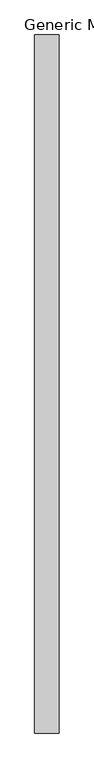
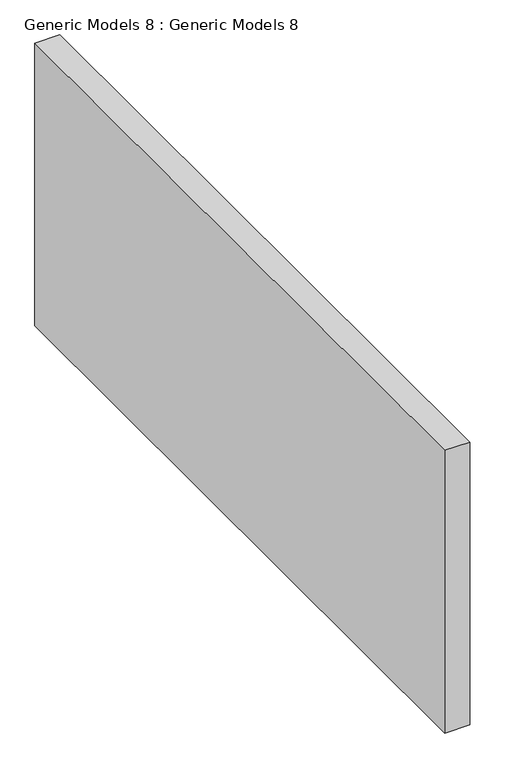
"""IFC4 building model written with IfcOpenShell, lengths in millimetres: proxy geometry, Generic Models 8 : Generic Models 8."""

from ifc_helpers import new_model, si_unit, frame, origin, place, context, project, spatial, polyline, outline, extrude, source, transform, mapped, element, save


def generic_models_8_generic_models_8_ec4d4fb3(model_context):
    return source(origin(), model_context, "Body", "SweptSolid", [
        extrude(outline(polyline([(-3185.3781265, -5887.8142532), (-3185.3781265, -4440.0142532), (-3134.5781265, -4440.0142532), (-3134.5781265, -5887.8142532), (-3185.3781265, -5887.8142532)])), frame((0.0, 0.0, 5791.2), z_axis=(0.0, 0.0, 1.0), x_axis=(1.0, 0.0, 0.0)), (0.0, 0.0, 1.0), 609.6),
    ])


if __name__ == "__main__":
    model = new_model("IFC4")
    model_context = context("Model", 3, world=origin())
    ifc_project = project(units=[si_unit("LENGTHUNIT", "METRE", prefix="MILLI")], contexts=[model_context])
    site = spatial("IfcSite", under=ifc_project)
    building = spatial("IfcBuilding", under=site)
    placement = place(None, origin())
    generic_models_8_generic_models_8_shape = generic_models_8_generic_models_8_ec4d4fb3(model_context)
    element("IfcBuildingElementProxy", 1, Name="Generic Models 8 : Generic Models 8", ObjectType="Generic Models 8 : Generic Models 8", at=placement, inside=building, context=model_context, shape_type="MappedRepresentation", body=[
        mapped(generic_models_8_generic_models_8_shape, transform((0.0, 0.0, 0.0), x_axis=(1.0, 0.0, 0.0), y_axis=(0.0, 1.0, 0.0), z_axis=(0.0, 0.0, 1.0))),
    ])
    save(model, "model.ifc")
